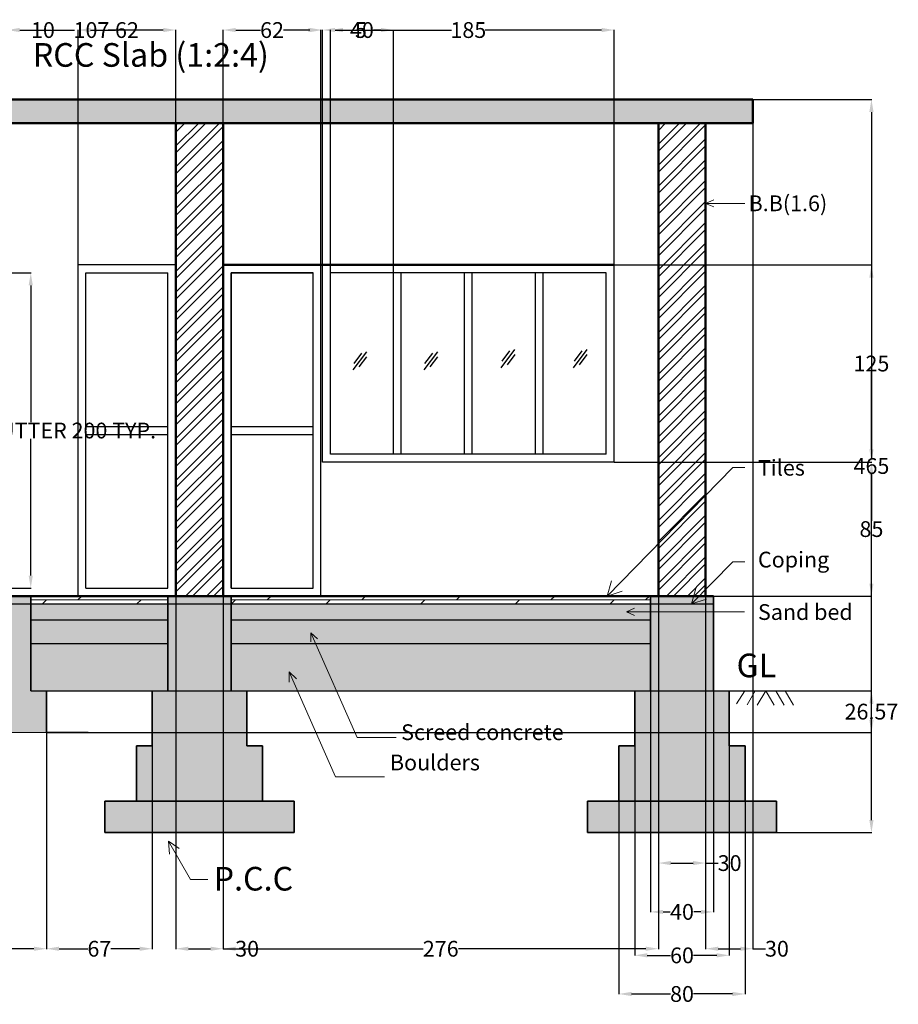
# Model space of a CAD drawing. Units: centimetres. Extents: x 1029 to 1924, y 29 to 653.
# Tile 2 of 2: x 1366 to 1924, y 29 to 653. Entities that reach past the tile are written whole.
import ezdxf

# ---------------------------------------------------------------- set-up
doc = ezdxf.new("R2010")
doc.units = ezdxf.units.CM
doc.header["$MEASUREMENT"] = 0
for name, color, linetype, lineweight in [('A-ANNO-DIMS', 2, 'Continuous', 18), ('A-ANNO-SYMB', 3, 'Continuous', 18), ('A-ANNO-TEXT', 7, 'Continuous', 18), ('A-DOOR', 4, 'Continuous', 25), ('A-FLOR', 3, 'Continuous', 25), ('A-FLOR-PATT', 252, 'Continuous', 13), ('A-GLAZ', 4, 'Continuous', 25), ('A-WALL', 7, 'Continuous', 50), ('A-WALL-PATT', 8, 'Continuous', 13), ('S-FNDN', 1, 'Continuous', 35), ('S-FNDN-PATT', 8, 'Continuous', 13), ('S-SLAB', 1, 'Continuous', 50)]:
    doc.layers.add(name, color=color, linetype=linetype, lineweight=lineweight)
doc.styles.get("Standard").update_dxf_attribs({"font": 'arial.ttf'})
doc.dimstyles.get("Standard").update_dxf_attribs({"dimtxt": 10, "dimasz": 7.98, "dimexe": 0.18, "dimexo": 0.0625, "dimgap": 0.09, "dimtad": 0, "dimtih": 1, "dimtoh": 1, "dimdec": 0, "dimzin": 0, "dimdsep": 46, "dimtxsty": 'Standard', "dimcen": 0.09, "dimadec": 0, "dimazin": 0, "dimtfac": 1, "dimtdec": 0, "dimtofl": 0, "dimtmove": 0, "dimatfit": 3, "dimfxl": 1, "dimtolj": 1, "dimtzin": 0, "dimarcsym": 0})
pattern_1 = [(50, (-21.744, 120), (14.345204, -1.25504), [1.5, -16.5]), (355, (-21.744, 120), (-2.77503, 15.04384), [1.2, -13.2]), (100.45144, (-20.549, 119.895), (11.57018, 13.7888), [1.2748, -14.02284]), (46.1842, (-21.744, 124), (21.34483, -3.31039), [2.25, -24.75]), (96.6356, (-19.965, 123.724), (18.69324, 19.48237), [1.9122, -21.03428]), (351.1842, (-21.744, 124), (18.69324, 19.48237), [1.8, -19.8]), (21, (-19.744, 123), (11.93814, -8.05238), [1.5, -16.5]), (326, (-19.744, 123), (4.86631, 14.503), [1.2, -13.2]), (71.45144, (-18.749, 122.329), (16.80445, 6.45062), [1.2748, -14.02284]), (37.5, (-21.744, 120), (0.243197, 6.657877), [0, -13.04, 0, -13.4, 0, -13.25]), (7.5, (-21.744, 120), (5.26139, 7.888234), [0, -7.64, 0, -12.74, 0, -5.05]), (327.5, (-26.204, 120), (10.676449, -0.451097), [0, -5, 0, -15.6, 0, -20.7]), (317.5, (-28.204, 120), (11.663723, 2.0021), [0, -6.5, 0, -10.36, 0, -14.7])]

# ---------------------------------------------------------------- blocks, each defined once
blk = doc.blocks.new('ARROW')
for p, q in [((1496.49, -12.2), (1482.5, 12.03)), ((1482.5, 12.03), (1483.1, 3.86)), ((1482.5, 12.03), (1489.28, 7.42)), ((1507.41, -12.2), (1496.49, -12.2))]:
    blk.add_line(p, q)
blk = doc.blocks.new('*D10')
at = {"layer": 'A-ANNO-DIMS', "color": 0, "lineweight": -2, "transparency": 16777216}
for p, q in [((1771.35, 287.4), (1771.35, 117.95)), ((1801.35, 287.4), (1801.35, 117.95)), ((1779.33, 118.13), (1793.37, 118.13)), ((1801.35, 118.13), (1809.33, 118.13))]:
    blk.add_line(p, q, dxfattribs=at)
at = {"layer": 'A-ANNO-DIMS', "color": 0, "transparency": 16777216}
for points in [[(1779.33, 119.46), (1779.33, 116.8), (1771.35, 118.13)], [(1793.37, 119.46), (1793.37, 116.8), (1801.35, 118.13)]]:
    blk.add_solid(points, dxfattribs=at)
at = {"layer": 'Defpoints', "color": 0, "transparency": 16777216}
for p in [(1771.35, 287.46), (1801.35, 287.46), (1801.35, 118.13)]:
    blk.add_point(p, dxfattribs=at)
at = {"layer": 'A-ANNO-DIMS', "color": 0, "transparency": 16777216, "insert": (1816.56, 118.13), "char_height": 10, "attachment_point": 5}
blk.add_mtext('\\A1;30', dxfattribs=at)
blk = doc.blocks.new('*D11')
at = {"layer": 'A-ANNO-DIMS', "color": 0, "lineweight": -2, "transparency": 16777216}
for p, q in [((1766.35, 227.4), (1766.35, 86.97)), ((1806.35, 227.4), (1806.35, 86.97)), ((1774.33, 87.15), (1778.91, 87.15)), ((1798.37, 87.15), (1793.78, 87.15))]:
    blk.add_line(p, q, dxfattribs=at)
at = {"layer": 'A-ANNO-DIMS', "color": 0, "transparency": 16777216}
for points in [[(1774.33, 88.48), (1774.33, 85.82), (1766.35, 87.15)], [(1798.37, 88.48), (1798.37, 85.82), (1806.35, 87.15)]]:
    blk.add_solid(points, dxfattribs=at)
at = {"layer": 'Defpoints', "color": 0, "transparency": 16777216}
for p in [(1766.35, 227.46), (1806.35, 227.46), (1806.35, 87.15)]:
    blk.add_point(p, dxfattribs=at)
at = {"layer": 'A-ANNO-DIMS', "color": 0, "transparency": 16777216, "insert": (1786.35, 87.15), "char_height": 10, "attachment_point": 5}
blk.add_mtext('\\A1;40', dxfattribs=at)
blk = doc.blocks.new('*D12')
at = {"layer": 'A-ANNO-DIMS', "color": 0, "lineweight": -2, "transparency": 16777216}
for p, q in [((1756.35, 227.4), (1756.35, 59.43)), ((1816.35, 227.4), (1816.35, 59.43)), ((1764.33, 59.61), (1779.08, 59.61)), ((1808.37, 59.61), (1793.61, 59.61))]:
    blk.add_line(p, q, dxfattribs=at)
at = {"layer": 'A-ANNO-DIMS', "color": 0, "transparency": 16777216}
for points in [[(1764.33, 60.94), (1764.33, 58.28), (1756.35, 59.61)], [(1808.37, 60.94), (1808.37, 58.28), (1816.35, 59.61)]]:
    blk.add_solid(points, dxfattribs=at)
at = {"layer": 'Defpoints', "color": 0, "transparency": 16777216}
for p in [(1756.35, 227.46), (1816.35, 227.46), (1816.35, 59.61)]:
    blk.add_point(p, dxfattribs=at)
at = {"layer": 'A-ANNO-DIMS', "color": 0, "transparency": 16777216, "insert": (1786.35, 59.61), "char_height": 10, "attachment_point": 5}
blk.add_mtext('\\A1;60', dxfattribs=at)
blk = doc.blocks.new('*D13')
at = {"layer": 'A-ANNO-DIMS', "color": 0, "lineweight": -2, "transparency": 16777216}
for p, q in [((1746.35, 192.4), (1746.35, 34.94)), ((1826.35, 192.4), (1826.35, 34.94)), ((1754.33, 35.12), (1779.1, 35.12)), ((1818.37, 35.12), (1793.59, 35.12))]:
    blk.add_line(p, q, dxfattribs=at)
at = {"layer": 'A-ANNO-DIMS', "color": 0, "transparency": 16777216}
for points in [[(1754.33, 36.45), (1754.33, 33.79), (1746.35, 35.12)], [(1818.37, 36.45), (1818.37, 33.79), (1826.35, 35.12)]]:
    blk.add_solid(points, dxfattribs=at)
at = {"layer": 'Defpoints', "color": 0, "transparency": 16777216}
for p in [(1746.35, 192.46), (1826.35, 192.46), (1826.35, 35.12)]:
    blk.add_point(p, dxfattribs=at)
at = {"layer": 'A-ANNO-DIMS', "color": 0, "transparency": 16777216, "insert": (1786.35, 35.12), "char_height": 10, "attachment_point": 5}
blk.add_mtext('\\A1;80', dxfattribs=at)
blk = doc.blocks.new('DOOR-SHUTTER-520')
for p, q in [((0, 200), (52, 200)), ((0, 97.5), (0, 200)), ((52, 97.5), (52, 200)), ((0, 102.5), (52, 102.5)), ((0, 0), (0, 97.5)), ((0, 97.5), (52, 97.5)), ((52, 0), (52, 97.5)), ((0, 0), (52, 0))]:
    blk.add_line(p, q)
blk = doc.blocks.new('GLASS-MARK')
for p, q in [((8.65, 11.48), (0, 0)), ((5.5, 10.62), (0.58, 4.09)), ((8.77, 8.32), (3.89, 1.84))]:
    blk.add_line(p, q)
blk = doc.blocks.new('*D16')
at = {"layer": 'A-ANNO-DIMS', "color": 0, "lineweight": -2, "transparency": 16777216}
for p, q in [((1343.41, 492.46), (1373.53, 492.46)), ((1373.35, 484.48), (1373.35, 397.73)), ((1373.35, 300.44), (1373.35, 387.2)), ((1343.41, 292.46), (1373.53, 292.46))]:
    blk.add_line(p, q, dxfattribs=at)
at = {"layer": 'A-ANNO-DIMS', "color": 0, "transparency": 16777216}
for points in [[(1372.02, 484.48), (1374.68, 484.48), (1373.35, 492.46)], [(1372.02, 300.44), (1374.68, 300.44), (1373.35, 292.46)]]:
    blk.add_solid(points, dxfattribs=at)
at = {"layer": 'Defpoints', "color": 0, "transparency": 16777216}
for p in [(1343.35, 492.46), (1373.35, 492.46), (1343.35, 292.46)]:
    blk.add_point(p, dxfattribs=at)
at = {"layer": 'A-ANNO-DIMS', "color": 0, "transparency": 16777216, "insert": (1373.35, 392.46), "char_height": 10, "attachment_point": 5}
blk.add_mtext('\\A1;DOOR SHUTTER 200 TYP.', dxfattribs=at)
blk = doc.blocks.new('*D21')
at = {"layer": 'A-ANNO-DIMS', "color": 0, "lineweight": -2, "transparency": 16777216}
for p, q in [((1340.37, 646.46), (1332.39, 646.46)), ((1348.35, 587.52), (1348.35, 646.64)), ((1358.35, 587.52), (1358.35, 646.64)), ((1366.33, 646.46), (1374.31, 646.46))]:
    blk.add_line(p, q, dxfattribs=at)
at = {"layer": 'A-ANNO-DIMS', "color": 0, "transparency": 16777216}
for points in [[(1340.37, 647.79), (1340.37, 645.13), (1348.35, 646.46)], [(1366.33, 647.79), (1366.33, 645.13), (1358.35, 646.46)]]:
    blk.add_solid(points, dxfattribs=at)
at = {"layer": 'Defpoints', "color": 0, "transparency": 16777216}
for p in [(1358.35, 646.46), (1348.35, 587.46), (1358.35, 587.46)]:
    blk.add_point(p, dxfattribs=at)
at = {"layer": 'A-ANNO-DIMS', "color": 0, "transparency": 16777216, "insert": (1381.07, 646.46), "char_height": 10, "attachment_point": 5}
blk.add_mtext('\\A1;10', dxfattribs=at)
blk = doc.blocks.new('*D22')
at = {"layer": 'A-ANNO-DIMS', "color": 0, "lineweight": -2, "transparency": 16777216}
for p, q in [((1358.35, 287.52), (1358.35, 646.64)), ((1366.33, 646.46), (1401.18, 646.46)), ((1457.37, 646.46), (1422.51, 646.46)), ((1465.35, 287.52), (1465.35, 646.64))]:
    blk.add_line(p, q, dxfattribs=at)
at = {"layer": 'A-ANNO-DIMS', "color": 0, "transparency": 16777216}
for points in [[(1366.33, 647.79), (1366.33, 645.13), (1358.35, 646.46)], [(1457.37, 647.79), (1457.37, 645.13), (1465.35, 646.46)]]:
    blk.add_solid(points, dxfattribs=at)
at = {"layer": 'Defpoints', "color": 0, "transparency": 16777216}
for p in [(1465.35, 646.46), (1358.35, 287.46), (1465.35, 287.46)]:
    blk.add_point(p, dxfattribs=at)
at = {"layer": 'A-ANNO-DIMS', "color": 0, "transparency": 16777216, "insert": (1411.85, 646.46), "char_height": 10, "attachment_point": 5}
blk.add_mtext('\\A1;107', dxfattribs=at)
blk = doc.blocks.new('*D23')
at = {"layer": 'A-ANNO-DIMS', "color": 0, "lineweight": -2, "transparency": 16777216}
for p, q in [((1465.35, 587.4), (1465.35, 63.62)), ((1495.35, 587.4), (1495.35, 63.62)), ((1473.33, 63.8), (1487.37, 63.8)), ((1495.35, 63.8), (1503.33, 63.8))]:
    blk.add_line(p, q, dxfattribs=at)
at = {"layer": 'A-ANNO-DIMS', "color": 0, "transparency": 16777216}
for points in [[(1473.33, 65.13), (1473.33, 62.47), (1465.35, 63.8)], [(1487.37, 65.13), (1487.37, 62.47), (1495.35, 63.8)]]:
    blk.add_solid(points, dxfattribs=at)
at = {"layer": 'Defpoints', "color": 0, "transparency": 16777216}
for p in [(1465.35, 587.46), (1495.35, 587.46), (1495.35, 63.8)]:
    blk.add_point(p, dxfattribs=at)
at = {"layer": 'A-ANNO-DIMS', "color": 0, "transparency": 16777216, "insert": (1510.56, 63.8), "char_height": 10, "attachment_point": 5}
blk.add_mtext('\\A1;30', dxfattribs=at)
blk = doc.blocks.new('*D24')
at = {"layer": 'A-ANNO-DIMS', "color": 0, "lineweight": -2, "transparency": 16777216}
for p, q in [((1495.35, 587.4), (1495.35, 63.62)), ((1771.35, 587.4), (1771.35, 63.62)), ((1503.33, 63.8), (1622.13, 63.8)), ((1763.37, 63.8), (1644.57, 63.8))]:
    blk.add_line(p, q, dxfattribs=at)
at = {"layer": 'A-ANNO-DIMS', "color": 0, "transparency": 16777216}
for points in [[(1503.33, 65.13), (1503.33, 62.47), (1495.35, 63.8)], [(1763.37, 65.13), (1763.37, 62.47), (1771.35, 63.8)]]:
    blk.add_solid(points, dxfattribs=at)
at = {"layer": 'Defpoints', "color": 0, "transparency": 16777216}
for p in [(1495.35, 587.46), (1771.35, 587.46), (1771.35, 63.8)]:
    blk.add_point(p, dxfattribs=at)
at = {"layer": 'A-ANNO-DIMS', "color": 0, "transparency": 16777216, "insert": (1633.35, 63.8), "char_height": 10, "attachment_point": 5}
blk.add_mtext('\\A1;276', dxfattribs=at)
blk = doc.blocks.new('*D25')
at = {"layer": 'A-ANNO-DIMS', "color": 0, "lineweight": -2, "transparency": 16777216}
for p, q in [((1801.35, 587.4), (1801.35, 63.62)), ((1831.35, 587.4), (1831.35, 63.62)), ((1809.33, 63.8), (1823.37, 63.8)), ((1831.35, 63.8), (1839.33, 63.8))]:
    blk.add_line(p, q, dxfattribs=at)
at = {"layer": 'A-ANNO-DIMS', "color": 0, "transparency": 16777216}
for points in [[(1809.33, 65.13), (1809.33, 62.47), (1801.35, 63.8)], [(1823.37, 65.13), (1823.37, 62.47), (1831.35, 63.8)]]:
    blk.add_solid(points, dxfattribs=at)
at = {"layer": 'Defpoints', "color": 0, "transparency": 16777216}
for p in [(1801.35, 587.46), (1831.35, 587.46), (1831.35, 63.8)]:
    blk.add_point(p, dxfattribs=at)
at = {"layer": 'A-ANNO-DIMS', "color": 0, "transparency": 16777216, "insert": (1846.56, 63.8), "char_height": 10, "attachment_point": 5}
blk.add_mtext('\\A1;30', dxfattribs=at)
blk = doc.blocks.new('*D28')
at = {"layer": 'A-ANNO-DIMS', "color": 0, "lineweight": -2, "transparency": 16777216}
for p, q in [((1403.35, 497.52), (1403.35, 646.64)), ((1411.33, 646.46), (1427.12, 646.46)), ((1457.37, 646.46), (1441.58, 646.46)), ((1465.35, 497.52), (1465.35, 646.64))]:
    blk.add_line(p, q, dxfattribs=at)
at = {"layer": 'A-ANNO-DIMS', "color": 0, "transparency": 16777216}
for points in [[(1411.33, 647.79), (1411.33, 645.13), (1403.35, 646.46)], [(1457.37, 647.79), (1457.37, 645.13), (1465.35, 646.46)]]:
    blk.add_solid(points, dxfattribs=at)
at = {"layer": 'Defpoints', "color": 0, "transparency": 16777216}
for p in [(1465.35, 646.46), (1403.35, 497.46), (1465.35, 497.46)]:
    blk.add_point(p, dxfattribs=at)
at = {"layer": 'A-ANNO-DIMS', "color": 0, "transparency": 16777216, "insert": (1434.35, 646.46), "char_height": 10, "attachment_point": 5}
blk.add_mtext('\\A1;62', dxfattribs=at)
blk = doc.blocks.new('*D29')
at = {"layer": 'A-ANNO-DIMS', "color": 0, "lineweight": -2, "transparency": 16777216}
for p, q in [((1495.35, 497.52), (1495.35, 646.64)), ((1503.33, 646.46), (1519.12, 646.46)), ((1549.37, 646.46), (1533.58, 646.46)), ((1557.35, 497.52), (1557.35, 646.64))]:
    blk.add_line(p, q, dxfattribs=at)
at = {"layer": 'A-ANNO-DIMS', "color": 0, "transparency": 16777216}
for points in [[(1503.33, 647.79), (1503.33, 645.13), (1495.35, 646.46)], [(1549.37, 647.79), (1549.37, 645.13), (1557.35, 646.46)]]:
    blk.add_solid(points, dxfattribs=at)
at = {"layer": 'Defpoints', "color": 0, "transparency": 16777216}
for p in [(1557.35, 646.46), (1495.35, 497.46), (1557.35, 497.46)]:
    blk.add_point(p, dxfattribs=at)
at = {"layer": 'A-ANNO-DIMS', "color": 0, "transparency": 16777216, "insert": (1526.35, 646.46), "char_height": 10, "attachment_point": 5}
blk.add_mtext('\\A1;62', dxfattribs=at)
blk = doc.blocks.new('*D30')
at = {"layer": 'A-ANNO-DIMS', "color": 0, "lineweight": -2, "transparency": 16777216}
for p, q in [((1558.35, 497.52), (1558.35, 646.64)), ((1566.33, 646.46), (1640.14, 646.46)), ((1735.37, 646.46), (1661.55, 646.46)), ((1743.35, 497.52), (1743.35, 646.64))]:
    blk.add_line(p, q, dxfattribs=at)
at = {"layer": 'A-ANNO-DIMS', "color": 0, "transparency": 16777216}
for points in [[(1566.33, 647.79), (1566.33, 645.13), (1558.35, 646.46)], [(1735.37, 647.79), (1735.37, 645.13), (1743.35, 646.46)]]:
    blk.add_solid(points, dxfattribs=at)
at = {"layer": 'Defpoints', "color": 0, "transparency": 16777216}
for p in [(1743.35, 646.46), (1558.35, 497.46), (1743.35, 497.46)]:
    blk.add_point(p, dxfattribs=at)
at = {"layer": 'A-ANNO-DIMS', "color": 0, "transparency": 16777216, "insert": (1650.85, 646.46), "char_height": 10, "attachment_point": 5}
blk.add_mtext('\\A1;185', dxfattribs=at)
blk = doc.blocks.new('*D31')
at = {"layer": 'A-ANNO-DIMS', "color": 0, "lineweight": -2, "transparency": 16777216}
for p, q in [((1550.37, 646.46), (1542.39, 646.46)), ((1558.35, 372.52), (1558.35, 646.64)), ((1563.35, 377.52), (1563.35, 646.64)), ((1571.33, 646.46), (1579.31, 646.46))]:
    blk.add_line(p, q, dxfattribs=at)
at = {"layer": 'A-ANNO-DIMS', "color": 0, "transparency": 16777216}
for points in [[(1550.37, 647.79), (1550.37, 645.13), (1558.35, 646.46)], [(1571.33, 647.79), (1571.33, 645.13), (1563.35, 646.46)]]:
    blk.add_solid(points, dxfattribs=at)
at = {"layer": 'Defpoints', "color": 0, "transparency": 16777216}
for p in [(1563.35, 646.46), (1563.35, 377.46), (1558.35, 372.46)]:
    blk.add_point(p, dxfattribs=at)
at = {"layer": 'A-ANNO-DIMS', "color": 0, "transparency": 16777216, "insert": (1582.71, 646.46), "char_height": 10, "attachment_point": 5}
blk.add_mtext('\\A1;5', dxfattribs=at)
blk = doc.blocks.new('*D32')
at = {"layer": 'A-ANNO-DIMS', "color": 0, "lineweight": -2, "transparency": 16777216}
for p, q in [((1563.35, 377.52), (1563.35, 646.64)), ((1571.33, 646.46), (1575.91, 646.46)), ((1595.37, 646.46), (1590.78, 646.46)), ((1603.35, 377.52), (1603.35, 646.64))]:
    blk.add_line(p, q, dxfattribs=at)
at = {"layer": 'A-ANNO-DIMS', "color": 0, "transparency": 16777216}
for points in [[(1571.33, 647.79), (1571.33, 645.13), (1563.35, 646.46)], [(1595.37, 647.79), (1595.37, 645.13), (1603.35, 646.46)]]:
    blk.add_solid(points, dxfattribs=at)
at = {"layer": 'Defpoints', "color": 0, "transparency": 16777216}
for p in [(1603.35, 646.46), (1563.35, 377.46), (1603.35, 377.46)]:
    blk.add_point(p, dxfattribs=at)
at = {"layer": 'A-ANNO-DIMS', "color": 0, "transparency": 16777216, "insert": (1583.35, 646.46), "char_height": 10, "attachment_point": 5}
blk.add_mtext('\\A1;40', dxfattribs=at)
blk = doc.blocks.new('*D33')
at = {"layer": 'A-ANNO-DIMS', "color": 0, "lineweight": -2, "transparency": 16777216}
for p, q in [((1743.41, 372.46), (1906.67, 372.46)), ((1906.49, 364.48), (1906.49, 335.16)), ((1906.49, 295.44), (1906.49, 324.77)), ((1738.87, 287.46), (1906.67, 287.46))]:
    blk.add_line(p, q, dxfattribs=at)
at = {"layer": 'A-ANNO-DIMS', "color": 0, "transparency": 16777216}
for points in [[(1905.16, 364.48), (1907.82, 364.48), (1906.49, 372.46)], [(1905.16, 295.44), (1907.82, 295.44), (1906.49, 287.46)]]:
    blk.add_solid(points, dxfattribs=at)
at = {"layer": 'Defpoints', "color": 0, "transparency": 16777216}
for p in [(1743.35, 372.46), (1906.49, 372.46), (1738.81, 287.46)]:
    blk.add_point(p, dxfattribs=at)
at = {"layer": 'A-ANNO-DIMS', "color": 0, "transparency": 16777216, "insert": (1906.49, 329.96), "char_height": 10, "attachment_point": 5}
blk.add_mtext('\\A1;85', dxfattribs=at)
blk = doc.blocks.new('*D34')
at = {"layer": 'A-ANNO-DIMS', "color": 0, "lineweight": -2, "transparency": 16777216}
for p, q in [((1743.41, 497.46), (1906.67, 497.46)), ((1906.49, 489.48), (1906.49, 440.16)), ((1906.49, 380.44), (1906.49, 429.77)), ((1743.41, 372.46), (1906.67, 372.46))]:
    blk.add_line(p, q, dxfattribs=at)
at = {"layer": 'A-ANNO-DIMS', "color": 0, "transparency": 16777216}
for points in [[(1905.16, 489.48), (1907.82, 489.48), (1906.49, 497.46)], [(1905.16, 380.44), (1907.82, 380.44), (1906.49, 372.46)]]:
    blk.add_solid(points, dxfattribs=at)
at = {"layer": 'Defpoints', "color": 0, "transparency": 16777216}
for p in [(1743.35, 497.46), (1906.49, 497.46), (1743.35, 372.46)]:
    blk.add_point(p, dxfattribs=at)
at = {"layer": 'A-ANNO-DIMS', "color": 0, "transparency": 16777216, "insert": (1906.49, 434.96), "char_height": 10, "attachment_point": 5}
blk.add_mtext('\\A1;125', dxfattribs=at)
blk = doc.blocks.new('*D43')
at = {"layer": 'A-ANNO-DIMS', "color": 0, "lineweight": -2, "transparency": 16777216}
for p, q in [((1323.35, 200.83), (1323.35, 63.62)), ((1383.35, 200.83), (1383.35, 63.62)), ((1331.33, 63.8), (1346.08, 63.8)), ((1375.37, 63.8), (1360.61, 63.8))]:
    blk.add_line(p, q, dxfattribs=at)
at = {"layer": 'A-ANNO-DIMS', "color": 0, "transparency": 16777216}
for points in [[(1331.33, 65.13), (1331.33, 62.47), (1323.35, 63.8)], [(1375.37, 65.13), (1375.37, 62.47), (1383.35, 63.8)]]:
    blk.add_solid(points, dxfattribs=at)
at = {"layer": 'Defpoints', "color": 0, "transparency": 16777216}
for p in [(1323.35, 200.89), (1383.35, 200.89), (1383.35, 63.8)]:
    blk.add_point(p, dxfattribs=at)
at = {"layer": 'A-ANNO-DIMS', "color": 0, "transparency": 16777216, "insert": (1353.35, 63.8), "char_height": 10, "attachment_point": 5}
blk.add_mtext('\\A1;60', dxfattribs=at)
blk = doc.blocks.new('*D44')
at = {"layer": 'A-ANNO-DIMS', "color": 0, "lineweight": -2, "transparency": 16777216}
for p, q in [((1383.35, 227.4), (1383.35, 63.62)), ((1450.35, 227.4), (1450.35, 63.62)), ((1391.33, 63.8), (1409.57, 63.8)), ((1442.37, 63.8), (1424.13, 63.8))]:
    blk.add_line(p, q, dxfattribs=at)
at = {"layer": 'A-ANNO-DIMS', "color": 0, "transparency": 16777216}
for points in [[(1391.33, 65.13), (1391.33, 62.47), (1383.35, 63.8)], [(1442.37, 65.13), (1442.37, 62.47), (1450.35, 63.8)]]:
    blk.add_solid(points, dxfattribs=at)
at = {"layer": 'Defpoints', "color": 0, "transparency": 16777216}
for p in [(1383.35, 227.46), (1450.35, 227.46), (1450.35, 63.8)]:
    blk.add_point(p, dxfattribs=at)
at = {"layer": 'A-ANNO-DIMS', "color": 0, "transparency": 16777216, "insert": (1416.85, 63.8), "char_height": 10, "attachment_point": 5}
blk.add_mtext('\\A1;67', dxfattribs=at)
blk = doc.blocks.new('*D45')
at = {"layer": 'A-ANNO-DIMS', "color": 0, "lineweight": -2, "transparency": 16777216}
for p, q in [((1383.41, 227.46), (1906.67, 227.46)), ((1906.49, 219.48), (1906.49, 219.37)), ((1906.49, 208.87), (1906.49, 208.98)), ((1383.41, 200.89), (1906.67, 200.89))]:
    blk.add_line(p, q, dxfattribs=at)
at = {"layer": 'A-ANNO-DIMS', "color": 0, "transparency": 16777216}
for points in [[(1905.16, 219.48), (1907.82, 219.48), (1906.49, 227.46)], [(1905.16, 208.87), (1907.82, 208.87), (1906.49, 200.89)]]:
    blk.add_solid(points, dxfattribs=at)
at = {"layer": 'Defpoints', "color": 0, "transparency": 16777216}
for p in [(1383.35, 227.46), (1383.35, 200.89), (1906.49, 200.89)]:
    blk.add_point(p, dxfattribs=at)
at = {"layer": 'A-ANNO-DIMS', "color": 0, "transparency": 16777216, "insert": (1906.49, 214.18), "char_height": 10, "attachment_point": 5}
blk.add_mtext('\\A1;26.57', dxfattribs=at)
blk = doc.blocks.new('*D46')
at = {"layer": 'A-ANNO-DIMS', "color": 0, "lineweight": -2, "transparency": 16777216}
for p, q in [((1831.41, 602.46), (1906.67, 602.46)), ((1906.49, 594.48), (1906.49, 375.16)), ((1906.49, 145.44), (1906.49, 364.77)), ((1846.41, 137.46), (1906.67, 137.46))]:
    blk.add_line(p, q, dxfattribs=at)
at = {"layer": 'A-ANNO-DIMS', "color": 0, "transparency": 16777216}
for points in [[(1905.16, 594.48), (1907.82, 594.48), (1906.49, 602.46)], [(1905.16, 145.44), (1907.82, 145.44), (1906.49, 137.46)]]:
    blk.add_solid(points, dxfattribs=at)
at = {"layer": 'Defpoints', "color": 0, "transparency": 16777216}
for p in [(1831.35, 602.46), (1846.35, 137.46), (1906.49, 137.46)]:
    blk.add_point(p, dxfattribs=at)
at = {"layer": 'A-ANNO-DIMS', "color": 0, "transparency": 16777216, "insert": (1906.49, 369.96), "char_height": 10, "attachment_point": 5}
blk.add_mtext('\\A1;465', dxfattribs=at)

msp = doc.modelspace()

# ---------------------------------------------------------------- hatches: boundary and pattern name
at = {"layer": 'A-FLOR-PATT'}
h = msp.add_hatch(dxfattribs=at)
h.set_pattern_fill('AR-CONC', color=256, scale=2)
h.set_pattern_definition(pattern_1)
h.paths.add_polyline_path([(1186.347, 287.462), (1186.347, 282.462), (1226.347, 282.462), (1226.347, 287.462)])
h.paths.add_polyline_path([(1373.347, 282.462), (1373.347, 287.462), (1333.347, 287.462), (1333.347, 282.462)])
h.paths.add_polyline_path([(1460.347, 287.462), (1460.347, 282.462), (1500.347, 282.462), (1500.347, 287.462)])
h.paths.add_polyline_path([(1766.347, 287.462), (1766.347, 282.462), (1806.347, 282.462), (1806.347, 287.462)])
h = msp.add_hatch(dxfattribs=at)
h.set_pattern_fill('DOLMIT', color=256, scale=20)
h.set_pattern_definition([(0, (-21.744, 120), (0, 5), []), (45, (-21.744, 120), (-10, 10), [7.07107, -14.14214])])
h.paths.add_polyline_path([(1333.347, 282.462), (1333.347, 287.462), (1226.347, 287.462), (1226.347, 282.462)])
h.paths.add_polyline_path([(1460.347, 282.462), (1460.347, 287.462), (1373.347, 287.462), (1373.347, 282.462)])
h.paths.add_polyline_path([(1766.347, 282.462), (1766.347, 287.462), (1500.347, 287.462), (1500.347, 282.462)])
h = msp.add_hatch(dxfattribs=at)
h.set_pattern_fill('ANSI33', color=256, scale=25)
h.set_pattern_definition([(45, (-21.744, 120), (-4.419417, 4.419417), []), (45, (-17.325, 120), (-4.419417, 4.419417), [3.125, -1.5625])])
h.paths.add_polyline_path([(1236.347, 227.462), (1226.347, 227.462), (1226.347, 282.462), (1186.347, 282.462), (1186.347, 227.462), (1176.347, 227.462), (1176.347, 192.462), (1166.347, 192.462), (1166.347, 157.462), (1246.347, 157.462), (1246.347, 192.462), (1236.347, 192.462)])
h.paths.add_polyline_path([(1510.347, 227.462), (1500.347, 227.462), (1500.347, 282.462), (1460.347, 282.462), (1460.347, 227.462), (1450.347, 227.462), (1450.347, 192.462), (1440.347, 192.462), (1440.347, 157.462), (1520.347, 157.462), (1520.347, 192.462), (1510.347, 192.462)])
h.paths.add_polyline_path([(1333.347, 227.462), (1323.347, 227.462), (1323.347, 200.892), (1349.035, 200.892), (1349.886, 204.258), (1349.886, 197.447), (1350.837, 200.892), (1383.347, 200.892), (1383.347, 227.462), (1373.347, 227.462), (1373.347, 282.462), (1333.347, 282.462)])
h.paths.add_polyline_path([(1756.347, 192.462), (1746.347, 192.462), (1746.347, 157.462), (1826.347, 157.462), (1826.347, 192.462), (1816.347, 192.462), (1816.347, 227.462), (1806.347, 227.462), (1806.347, 282.462), (1766.347, 282.462), (1766.347, 227.462), (1756.347, 227.462)])
h = msp.add_hatch(dxfattribs=at)
h.set_pattern_fill('AR-SAND', color=256, scale=5)
h.set_pattern_definition([(37.5, (-21.744, 120), (-0.314967, 9.63412), [0, -7.6, 0, -8.5, 0, -8.125]), (7.5, (-21.744, 120), (8.84888, 14.11073), [0, -4.1, 0, -6.85, 0, -2.625]), (327.5, (-27.894, 120), (15.57071, 0.028295), [0, -2.5, 0, -9, 0, -11.75]), (317.5, (-27.894, 120), (15.03063, 4.38838), [0, -1.25, 0, -5.9, 0, -6.75])])
h.paths.add_polyline_path([(1226.347, 282.462), (1226.347, 272.462), (1333.347, 272.462), (1333.347, 282.462)])
h.paths.add_polyline_path([(1460.347, 272.462), (1460.347, 282.462), (1373.347, 282.462), (1373.347, 272.462)])
h.paths.add_polyline_path([(1766.347, 272.462), (1766.347, 282.462), (1500.347, 282.462), (1500.347, 272.462)])
h = msp.add_hatch(dxfattribs=at)
h.set_pattern_fill('GRAVEL', color=256, scale=20)
h.set_pattern_definition([(228.01279, (-7.3441, 140), (-160, -180), [2.69072, -266.38176]), (184.96974, (-9.14414, 138), (240, 20), [4.61736, -457.1185]), (132.51045, (-13.7441, 137.6), (200, -220), [3.25576, -322.32065]), (267.27369, (-21.5441, 132.6), (20, 400), [4.20476, -416.27116]), (292.833654, (-21.7441, 128.4), (-100, 240), [4.1231, -408.18746]), (357.27369, (-20.1441, 124.6), (-400, 20), [4.20476, -416.27116]), (37.69424, (-15.94414, 124.4), (-260, -200), [5.56058, -550.49697]), (72.25533, (-11.54414, 127.8), (140, 440), [5.24976, -519.72643]), (121.429566, (-9.9441, 132.8), (-160, 260), [4.219, -417.68146]), (175.23636, (-12.1441, 136.4), (220, -20), [4.81664, -236.01525]), (222.397438, (-16.94414, 136.8), (-240, -220), [6.22896, -616.6675]), (138.81407, (-1.7441, 132.4), (-140, 120), [2.12602, -210.4769]), (171.469234, (-3.3441, 133.8), (260, -40), [4.04474, -400.43023]), (225, (-7.344, 134.4), (-2e-15, -20), [2.82842, -25.45585]), (203.19859, (-8.7441, 136.8), (100, 40), [1.52316, -150.7923]), (291.8014, (-10.144, 136.2), (-20, 60), [2.15406, -105.54924]), (30.96376, (-9.344, 134.2), (60, 40), [3.49858, -113.12046]), (161.56505, (-6.344, 136), (40, -20), [2.52982, -60.71573]), (16.38954, (-21.7441, 136.2), (200, 60), [3.544, -350.8569]), (70.34618, (-18.3441, 137.2), (-80, -220), [2.97322, -294.34815]), (293.19859, (-6.3441, 140), (-40, 100), [3.0463, -149.26916]), (343.61046, (-5.1441, 137.2), (-200, 60), [3.544, -350.8569]), (339.44395, (-21.7441, 123.8), (-100, 40), [3.4176, -167.46247]), (294.77514, (-18.5441, 122.6), (-100, 220), [2.86356, -283.49286]), (66.80141, (-6.1441, 120), (40, 100), [3.0463, -149.26916]), (17.354025, (-4.9441, 122.8), (-260, -80), [3.35262, -331.90847]), (69.44395, (-15.9441, 120), (-40, -100), [1.7088, -169.17127]), (101.30993, (-7.344, 120), (-20, 80), [1.0198, -100.9606]), (165.96376, (-7.544, 121), (60, -20), [4.1231, -78.33901]), (186.009006, (-11.5441, 122), (200, 20), [3.821, -378.27846]), (303.69007, (-9.344, 132.4), (-20, 40), [2.88444, -69.22659]), (353.157227, (-7.74414, 130), (340, -40), [5.03588, -498.55125]), (60.9454, (-2.7441, 129.4), (-80, -140), [2.05912, -203.85348]), (90, (-1.744, 131.2), (-20, 20), [1.2, -18.8]), (120.25644, (-11.9441, 122.6), (80, -140), [2.77848, -275.0704]), (48.01279, (-13.3441, 125), (160, 180), [5.38144, -263.69104]), (0, (-9.744, 129), (20, 20), [5.2, -14.8]), (325.30485, (-4.5441, 129), (200, -140), [3.16228, -313.06549]), (254.0546, (-1.9441, 127.2), (-20, -80), [2.91204, -142.69016]), (207.645975, (-2.74414, 124.4), (-380, -200), [4.7413, -469.38948]), (175.42608, (-6.94414, 122.2), (-260, 20), [5.01598, -496.58147])])
h.paths.add_polyline_path([(1226.347, 257.462), (1226.347, 227.462), (1236.347, 227.462), (1333.347, 227.462), (1333.347, 257.462)])
h.paths.add_polyline_path([(1460.347, 227.462), (1460.347, 257.462), (1373.347, 257.462), (1373.347, 227.462)])
h.paths.add_polyline_path([(1756.347, 227.462), (1766.347, 227.462), (1766.347, 257.462), (1500.347, 257.462), (1500.347, 227.462)])
at = {"layer": 'A-WALL-PATT'}
h = msp.add_hatch(dxfattribs=at)
h.set_pattern_fill('AR-CONC', color=256, scale=2)
h.set_pattern_definition(pattern_1)
h.paths.add_polyline_path([(1831.347, 587.462), (1831.347, 602.462), (1161.347, 602.462), (1161.347, 587.462)])
h.paths.add_polyline_path([(1460.347, 257.462), (1460.347, 272.462), (1373.347, 272.462), (1373.347, 257.462)])
h.paths.add_polyline_path([(1333.347, 257.462), (1333.347, 272.462), (1226.347, 272.462), (1226.347, 257.462)])
h.paths.add_polyline_path([(1766.347, 257.462), (1766.347, 272.462), (1500.347, 272.462), (1500.347, 257.462)])
h = msp.add_hatch(dxfattribs=at)
h.set_pattern_fill('ANSI32', color=256, scale=25)
h.set_pattern_definition([(45, (-21.744, 120), (-6.629126, 6.629126), []), (45, (-17.325, 120), (-6.629126, 6.629126), [])])
h.paths.add_polyline_path([(1221.347, 497.462), (1191.347, 497.462), (1191.347, 287.462), (1221.347, 287.462)])
h.paths.add_polyline_path([(1348.347, 287.462), (1358.347, 287.462), (1358.347, 587.462), (1348.347, 587.462)])
h.paths.add_polyline_path([(1495.347, 587.462), (1465.347, 587.462), (1465.347, 287.462), (1495.347, 287.462)])
h.paths.add_polyline_path([(1771.347, 287.462), (1801.347, 287.462), (1801.347, 587.462), (1771.347, 587.462)])
h.paths.add_polyline_path([(1221.347, 587.462), (1191.347, 587.462), (1191.347, 557.462), (1221.347, 557.462)])
at = {"layer": 'S-FNDN-PATT'}
h = msp.add_hatch(dxfattribs=at)
h.set_pattern_fill('AR-CONC', color=256, scale=2)
h.set_pattern_definition(pattern_1)
h.paths.add_polyline_path([(1146.347, 157.462), (1146.347, 137.462), (1266.347, 137.462), (1266.347, 157.462)])
h.paths.add_polyline_path([(1540.347, 137.462), (1540.347, 157.462), (1420.347, 157.462), (1420.347, 137.462)])
h.paths.add_polyline_path([(1846.347, 137.462), (1846.347, 157.462), (1726.347, 157.462), (1726.347, 137.462)])

# ---------------------------------------------------------------- linework, layer by layer
at = {"layer": 'A-ANNO-SYMB'}
for p, q in [((1801.347, 536.543), (1806.571, 538.814)), ((1801.347, 536.543), (1826.126, 536.493)), ((1801.347, 536.543), (1806.562, 534.251)), ((1738.806, 287.462), (1818.668, 369.021)), ((1818.668, 369.021), (1826.126, 369.021)), ((1792.279, 282.462), (1818.547, 309.288)), ((1818.547, 309.288), (1826.126, 309.288)), ((1738.806, 287.462), (1741.672, 297.173)), ((1738.806, 287.462), (1748.455, 290.531)), ((1792.279, 282.462), (1795.145, 292.173)), ((1792.279, 282.462), (1801.928, 285.531)), ((1751.077, 277.433), (1756.3, 279.704)), ((1751.077, 277.433), (1826.069, 277.433)), ((1751.077, 277.433), (1756.291, 275.142)), ((1550.95, 264.128), (1580.361, 197.676)), ((1550.95, 264.128), (1550.976, 258.432)), ((1550.95, 264.128), (1555.148, 260.279)), ((1537.233, 239.344), (1566.645, 172.891)), ((1537.233, 239.344), (1537.233, 232.959)), ((1537.233, 239.344), (1541.959, 235.051)), ((1826.241, 227.462), (1820.992, 219.091)), ((1832.776, 227.462), (1827.627, 218.398)), ((1839.419, 227.462), (1834.068, 218.195)), ((1839.419, 227.462), (1844.769, 218.195)), ((1845.848, 227.462), (1851.198, 218.195)), ((1851.69, 227.462), (1857.041, 218.195)), ((1350.837, 200.892), (1383.347, 200.892)), ((1580.361, 197.676), (1605.178, 197.676)), ((1566.645, 172.891), (1597.607, 172.891))]:
    msp.add_line(p, q, dxfattribs=at)
at = {"layer": 'A-DOOR'}
for p, q in [((1403.347, 287.462), (1403.347, 497.462)), ((1465.347, 497.462), (1403.347, 497.462)), ((1557.347, 287.462), (1557.347, 497.462)), ((1500.347, 492.462), (1500.347, 292.462)), ((1552.347, 492.462), (1500.347, 492.462))]:
    msp.add_line(p, q, dxfattribs=at)
at = {"layer": 'A-FLOR'}
for p, q in [((1186.347, 282.462), (1373.347, 282.462)), ((1373.347, 282.462), (1806.347, 282.462)), ((1373.347, 272.462), (1460.347, 272.462)), ((1500.347, 272.462), (1766.347, 272.462)), ((1373.347, 257.462), (1460.347, 257.462)), ((1500.347, 257.462), (1766.347, 257.462)), ((1373.347, 227.462), (1460.347, 227.462)), ((1450.347, 227.462), (1460.347, 227.462)), ((1500.347, 227.462), (1510.347, 227.462)), ((1500.347, 227.462), (1756.347, 227.462)), ((1756.347, 227.462), (1766.347, 227.462)), ((1806.347, 227.462), (1816.347, 227.462)), ((1816.347, 227.462), (1862.49, 227.462))]:
    msp.add_line(p, q, dxfattribs=at)
at = {"layer": 'A-GLAZ'}
for p, q in [((1558.347, 372.462), (1558.347, 497.462)), ((1743.347, 372.462), (1743.347, 497.462)), ((1738.347, 492.462), (1563.347, 492.462)), ((1563.347, 377.462), (1563.347, 492.462)), ((1603.347, 377.462), (1603.347, 492.462)), ((1608.347, 377.462), (1608.347, 492.462)), ((1648.347, 377.462), (1648.347, 492.462)), ((1653.347, 377.462), (1653.347, 492.462)), ((1693.347, 377.462), (1693.347, 492.462)), ((1698.347, 377.462), (1698.347, 492.462)), ((1738.347, 377.462), (1738.347, 492.462)), ((1738.347, 377.462), (1563.347, 377.462)), ((1743.347, 372.462), (1558.347, 372.462))]:
    msp.add_line(p, q, dxfattribs=at)
at = {"layer": 'A-WALL'}
for p, q in [((1465.347, 587.462), (1465.347, 287.462)), ((1495.347, 587.462), (1495.347, 287.462)), ((1771.347, 587.462), (1771.347, 287.462)), ((1801.347, 587.462), (1801.347, 287.462)), ((1743.347, 497.462), (1495.347, 497.462)), ((1226.347, 287.462), (1766.347, 287.462)), ((1333.347, 287.462), (1373.347, 287.462)), ((1460.347, 287.462), (1500.347, 287.462)), ((1766.347, 287.462), (1806.347, 287.462))]:
    msp.add_line(p, q, dxfattribs=at)
at = {"layer": 'S-FNDN'}
for p, q in [((1373.347, 227.462), (1373.347, 287.462)), ((1460.347, 287.462), (1460.347, 227.462)), ((1500.347, 287.462), (1500.347, 227.462)), ((1766.347, 287.462), (1766.347, 227.462)), ((1806.347, 287.462), (1806.347, 227.462)), ((1383.347, 227.462), (1383.347, 200.892)), ((1450.347, 227.462), (1450.347, 192.462)), ((1450.347, 227.462), (1450.347, 192.462)), ((1510.347, 227.462), (1510.347, 192.462)), ((1510.347, 227.462), (1510.347, 192.462)), ((1756.347, 227.462), (1756.347, 192.462)), ((1816.347, 227.462), (1816.347, 192.462)), ((1816.347, 227.462), (1816.347, 192.462)), ((1383.347, 200.892), (1409.652, 200.892)), ((1440.347, 192.462), (1440.347, 157.462)), ((1440.347, 192.462), (1450.347, 192.462)), ((1510.347, 192.462), (1520.347, 192.462)), ((1520.347, 192.462), (1520.347, 157.462)), ((1746.347, 192.462), (1746.347, 157.462)), ((1746.347, 192.462), (1756.347, 192.462)), ((1816.347, 192.462), (1826.347, 192.462)), ((1826.347, 192.462), (1826.347, 157.462)), ((1420.347, 157.462), (1420.347, 137.462)), ((1420.347, 157.462), (1540.347, 157.462)), ((1540.347, 157.462), (1540.347, 137.462)), ((1726.347, 157.462), (1726.347, 137.462)), ((1726.347, 157.462), (1846.347, 157.462)), ((1846.347, 157.462), (1846.347, 137.462)), ((1420.347, 137.462), (1540.347, 137.462)), ((1726.347, 137.462), (1846.347, 137.462))]:
    msp.add_line(p, q, dxfattribs=at)
at = {"layer": 'S-SLAB'}
for p, q in [((1161.347, 602.462), (1831.347, 602.462)), ((1831.347, 602.462), (1831.347, 587.462)), ((1161.347, 587.462), (1831.347, 587.462)), ((1465.347, 587.462), (1495.347, 587.462)), ((1771.347, 587.462), (1801.347, 587.462))]:
    msp.add_line(p, q, dxfattribs=at)

# ---------------------------------------------------------------- block references
at = {"layer": 'A-ANNO-SYMB'}
msp.add_blockref('ARROW', (-21.744, 120), dxfattribs=at)
at = {"layer": 'A-DOOR'}
for p in [(1408.347, 292.462), (1500.347, 292.462)]:
    msp.add_blockref('DOOR-SHUTTER-520', p, dxfattribs=at)
at = {"layer": 'A-GLAZ'}
for p in [(1671.544, 432.287), (1717.317, 432.287), (1577.574, 430.941), (1622.539, 430.941)]:
    msp.add_blockref('GLASS-MARK', p, dxfattribs=at)

# ---------------------------------------------------------------- texts
at = {"layer": 'A-ANNO-TEXT', "attachment_point": 1}
for s, width, insert, char_height in [('RCC Slab (1:2:4)', 292.57993, (1374.611, 638.174), 15), ('B.B(1.6)', 73.75091, (1828.583, 541.571), 10), ('Tiles', 144.15997, (1834.527, 373.868), 10), ('Coping', 144.15997, (1834.527, 315.595), 10), ('Sand bed', 144.15997, (1834.527, 282.339), 10), ('GL', 79.22541, (1820.97, 250.98), 15), ('Screed concrete ', 109.18888, (1608.237, 206.133), 10), ('Boulders', 79.22541, (1601.112, 186.929), 10), ('P.C.C', 79.22541, (1489.324, 115.712), 15)]:
    msp.add_mtext_dynamic_manual_height_columns(s, width=width, gutter_width=1, heights=[0], dxfattribs=dict(at, insert=insert, char_height=char_height))

# ---------------------------------------------------------------- dimensions: what is measured, and where the dimension line sits
at = {"layer": 'A-ANNO-DIMS'}
for base, p1, p2, picture, middle in [((1358.347, 646.462), (1348.347, 587.462), (1358.347, 587.462), '*D21', (1381.072, 646.462)), ((1465.347, 646.462), (1358.347, 287.462), (1465.347, 287.462), '*D22', (1411.847, 646.462)), ((1465.347, 646.462), (1403.347, 497.462), (1465.347, 497.462), '*D28', (1434.347, 646.462)), ((1557.347, 646.462), (1495.347, 497.462), (1557.347, 497.462), '*D29', (1526.347, 646.462)), ((1563.347, 646.462), (1558.347, 372.462), (1563.347, 377.462), '*D31', (1582.712, 646.462)), ((1743.347, 646.462), (1558.347, 497.462), (1743.347, 497.462), '*D30', (1650.847, 646.462)), ((1603.347, 646.462), (1563.347, 377.462), (1603.347, 377.462), '*D32', (1583.347, 646.462)), ((1495.347, 63.803), (1465.347, 587.462), (1495.347, 587.462), '*D23', (1510.559, 63.803)), ((1771.347, 63.803), (1495.347, 587.462), (1771.347, 587.462), '*D24', (1633.347, 63.803)), ((1831.347, 63.803), (1801.347, 587.462), (1831.347, 587.462), '*D25', (1846.559, 63.803)), ((1450.347, 63.803), (1383.347, 227.462), (1450.347, 227.462), '*D44', (1416.847, 63.803)), ((1383.347, 63.803), (1323.347, 200.892), (1383.347, 200.892), '*D43', (1353.347, 63.803))]:
    dim = msp.add_linear_dim(base=base, p1=p1, p2=p2, dimstyle='Standard', override={"dimdec": 0, "dimlfac": 1, "dimrnd": 0, "dimzin": 0, "dimdsep": 46, "dimlunit": 2}, dxfattribs=at)
    dim.commit()
    dim.dimension.update_dxf_attribs({"geometry": picture, "text_midpoint": middle})
for base, p1, p2, override, picture, middle in [((1906.49, 137.462), (1831.347, 602.462), (1846.347, 137.462), {"dimdec": 0, "dimlfac": 1, "dimrnd": 0, "dimzin": 0, "dimdsep": 46, "dimlunit": 2}, '*D46', (1906.49, 369.962)), ((1906.49, 497.462), (1743.347, 372.462), (1743.347, 497.462), {"dimdec": 0, "dimlfac": 1, "dimrnd": 0, "dimzin": 0, "dimdsep": 46, "dimlunit": 2}, '*D34', (1906.49, 434.962)), ((1906.49, 372.462), (1738.806, 287.462), (1743.347, 372.462), {"dimdec": 0, "dimlfac": 1, "dimrnd": 0, "dimzin": 0, "dimdsep": 46, "dimlunit": 2}, '*D33', (1906.49, 329.962)), ((1906.49, 200.892), (1383.347, 227.462), (1383.347, 200.892), {"dimdec": 2, "dimlfac": 1, "dimrnd": 0, "dimzin": 0, "dimdsep": 46, "dimlunit": 2}, '*D45', (1906.49, 214.177))]:
    dim = msp.add_linear_dim(base=base, p1=p1, p2=p2, angle=90, dimstyle='Standard', override=override, dxfattribs=at)
    dim.commit()
    dim.dimension.update_dxf_attribs({"geometry": picture, "text_midpoint": middle})
dim = msp.add_linear_dim(base=(1373.347, 492.462), p1=(1343.347, 292.462), p2=(1343.347, 492.462), angle=90, text='DOOR SHUTTER <> TYP.', dimstyle='Standard', override={"dimdec": 0, "dimlfac": 1, "dimrnd": 0, "dimzin": 0, "dimdsep": 46, "dimlunit": 2}, dxfattribs=at)
dim.commit()
dim.dimension.update_dxf_attribs({"geometry": '*D16', "text_midpoint": (1373.347, 392.462)})
for p1, p2, distance, picture, middle in [((1771.347, 287.462), (1801.347, 287.462), -169.337, '*D10', (1816.559, 118.125)), ((1756.347, 227.462), (1816.347, 227.462), -167.852, '*D12', (1786.347, 59.61)), ((1766.347, 227.462), (1806.347, 227.462), -140.312, '*D11', (1786.347, 87.15)), ((1746.347, 192.462), (1826.347, 192.462), -157.342, '*D13', (1786.347, 35.12))]:
    dim = msp.add_aligned_dim(p1=p1, p2=p2, distance=distance, dimstyle='Standard', override={"dimclrd": 0, "dimclre": 0, "dimclrt": 0}, dxfattribs=at)
    dim.commit()
    dim.dimension.update_dxf_attribs({"geometry": picture, "text_midpoint": middle})

doc.saveas('drawing.dxf')
